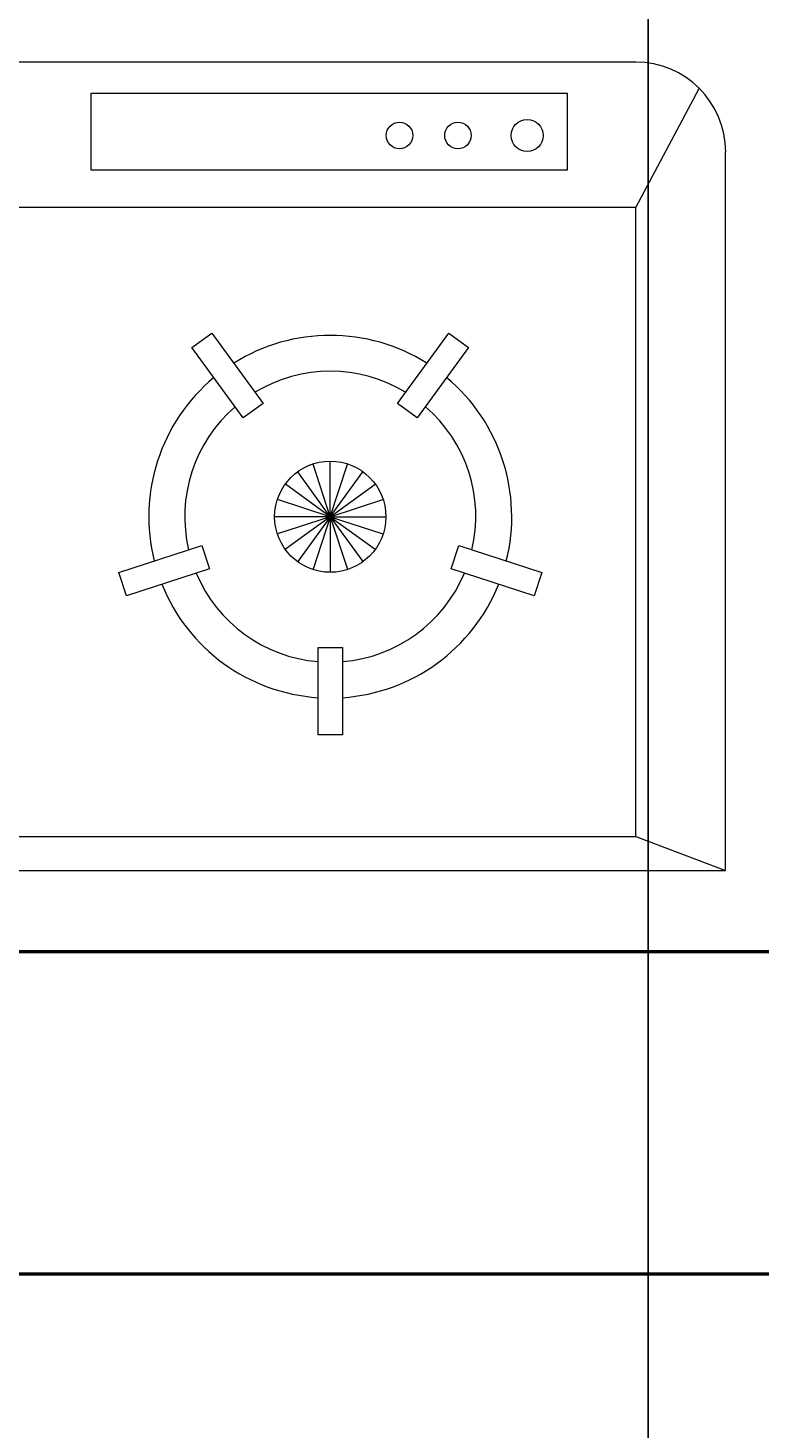
# Model space of a CAD drawing. Units: inches. Extents: x -173 to 545, y -746 to 104.
# Tile 5 of 32: x 203 to 223, y -702 to -663. Entities that reach past the tile are written whole.
import ezdxf

# ---------------------------------------------------------------- set-up
doc = ezdxf.new("R2010")
doc.units = ezdxf.units.IN
doc.header["$MEASUREMENT"] = 0
for name, color, linetype, lineweight in [('A-ANNO-DIMS', 2, 'Continuous', 18), ('A-EQPM', 8, 'Continuous', 18), ('A-WALL', 7, 'Continuous', 50)]:
    doc.layers.add(name, color=color, linetype=linetype, lineweight=lineweight)
doc.styles.get("Standard").update_dxf_attribs({"font": 'arial.ttf'})
doc.dimstyles.get("Standard").update_dxf_attribs({"dimtxt": 0.18, "dimasz": 0.18, "dimexe": 0.18, "dimexo": 0.0625, "dimgap": 0.09, "dimtad": 0, "dimtih": 1, "dimtoh": 1, "dimdec": 0, "dimzin": 0, "dimdsep": 46, "dimlunit": 3, "dimtxsty": 'Standard', "dimcen": 0.09, "dimadec": 0, "dimazin": 0, "dimtfac": 1, "dimtdec": 0, "dimtofl": 0, "dimtmove": 0, "dimatfit": 3, "dimfxl": 1, "dimtolj": 1, "dimtzin": 0, "dimarcsym": 0})

# ---------------------------------------------------------------- blocks, each defined once
blk = doc.blocks.new('HOB-40-BURNER')
for p, q in [((2.04, 10.813), (2.594, 11.215)), ((2.594, 11.215), (4.025, 9.246)), ((7.767, 9.246), (9.198, 11.215)), ((9.198, 11.215), (9.752, 10.813)), ((3.471, 8.844), (2.04, 10.813)), ((9.752, 10.813), (8.321, 8.844)), ((4.025, 9.246), (3.471, 8.844)), ((8.321, 8.844), (7.767, 9.246)), ((5.896, 6.088), (5.419, 7.557)), ((5.896, 6.088), (5.896, 7.633)), ((5.896, 6.088), (6.373, 7.557)), ((5.896, 6.088), (4.988, 7.338)), ((5.896, 6.088), (6.804, 7.338)), ((5.896, 6.088), (4.647, 6.996)), ((5.896, 6.088), (7.145, 6.996)), ((5.896, 6.088), (4.428, 6.566)), ((5.896, 6.088), (7.365, 6.566)), ((5.896, 6.088), (4.352, 6.088)), ((5.896, 6.088), (4.428, 5.611)), ((5.896, 6.088), (4.647, 5.181)), ((5.896, 6.088), (4.988, 4.839)), ((5.896, 6.088), (5.419, 4.62)), ((5.896, 6.088), (7.44, 6.088)), ((5.896, 6.088), (7.365, 5.611)), ((5.896, 6.088), (7.145, 5.181)), ((5.896, 6.088), (6.804, 4.839)), ((5.896, 6.088), (6.373, 4.62)), ((5.896, 6.088), (5.896, 4.544)), ((0, 4.532), (2.315, 5.285)), ((2.315, 5.285), (2.527, 4.634)), ((9.266, 4.634), (9.477, 5.285)), ((9.477, 5.285), (11.792, 4.532)), ((0.211, 3.882), (0, 4.532)), ((2.527, 4.634), (0.211, 3.882)), ((11.581, 3.882), (9.266, 4.634)), ((11.792, 4.532), (11.581, 3.882)), ((5.554, 2.434), (6.238, 2.434)), ((5.554, 0), (5.554, 2.434)), ((6.238, 2.434), (6.238, 0)), ((6.238, 0), (5.554, 0))]:
    blk.add_line(p, q)
blk.add_circle((5.896, 6.088), 1.551)
for radius, start, end in [(5.061, 57.8765, 122.1235), (5.061, 129.8765, 194.1235), (4.058, 58.8365, 121.1635), (5.061, 345.8765, 50.1235), (4.058, 130.8365, 193.1635), (4.058, 346.8365, 49.1635), (4.058, 202.8365, 265.1635), (4.058, 274.8365, 337.1635), (5.061, 201.8765, 266.1235), (5.061, 273.8765, 338.1235)]:
    blk.add_arc((5.896, 6.088), radius, start, end)
blk = doc.blocks.new('*D81')
at = {"layer": 'A-ANNO-DIMS', "color": 0, "lineweight": -2, "transparency": 16777216}
for p, q in [((219.801, -551.924), (219.801, -740.642)), ((306.301, -551.924), (306.301, -740.642)), ((219.981, -740.462), (262.513, -740.462)), ((306.121, -740.462), (263.59, -740.462))]:
    blk.add_line(p, q, dxfattribs=at)
at = {"layer": 'A-ANNO-DIMS', "color": 0, "transparency": 16777216}
for points in [[(219.981, -740.432), (219.981, -740.492), (219.801, -740.462)], [(306.121, -740.432), (306.121, -740.492), (306.301, -740.462)]]:
    blk.add_solid(points, dxfattribs=at)
at = {"layer": 'Defpoints', "color": 0, "transparency": 16777216}
for p in [(219.801, -551.862), (306.301, -551.862), (306.301, -740.462)]:
    blk.add_point(p, dxfattribs=at)
at = {"layer": 'A-ANNO-DIMS', "color": 0, "transparency": 16777216, "insert": (263.051, -740.462), "char_height": 0.18, "attachment_point": 5}
blk.add_mtext('\\A1;7\'-2 1/2"', dxfattribs=at)

msp = doc.modelspace()

# ---------------------------------------------------------------- linework, layer by layer
at = {"layer": 'A-EQPM'}
for p, q in [((219.455, -663.545), (184.36, -663.545)), ((204.268, -664.408), (217.538, -664.408)), ((204.268, -666.557), (204.268, -664.408)), ((217.538, -664.408), (217.538, -666.557)), ((219.455, -667.606), (221.227, -664.279)), ((221.961, -686.106), (221.961, -666.052)), ((217.538, -666.557), (204.268, -666.557)), ((219.455, -667.606), (184.36, -667.606)), ((219.455, -685.154), (219.455, -667.606)), ((184.36, -685.154), (219.455, -685.154)), ((219.455, -685.154), (221.961, -686.106)), ((181.854, -686.106), (221.961, -686.106))]:
    msp.add_line(p, q, dxfattribs=at)
for centre, radius in [((212.867, -665.593), 0.37), ((214.498, -665.593), 0.37), ((216.426, -665.593), 0.445)]:
    msp.add_circle(centre, radius, dxfattribs=at)
msp.add_arc((219.455, -666.052), 2.507, 0, 90, dxfattribs=at)
at = {"layer": 'A-WALL'}
for p, q in [((169.801, -688.362), (260.801, -688.362)), ((24.301, -697.362), (501.801, -697.362))]:
    msp.add_line(p, q, dxfattribs=at)

# ---------------------------------------------------------------- block references
at = {"layer": 'A-EQPM'}
msp.add_blockref('HOB-40-BURNER', (205.041, -682.32), dxfattribs=at)

# ---------------------------------------------------------------- dimensions: what is measured, and where the dimension line sits
at = {"layer": 'A-ANNO-DIMS'}
dim = msp.add_linear_dim(base=(306.301, -740.462), p1=(219.801, -551.862), p2=(306.301, -551.862), dimstyle='Standard', override={"dimdec": 1, "dimlfac": 1, "dimrnd": 0, "dimzin": 1, "dimdsep": 46, "dimlunit": 4, "dimfrac": 2}, dxfattribs=at)
dim.commit()
dim.dimension.update_dxf_attribs({"geometry": '*D81', "text_midpoint": (263.051, -740.462)})

doc.saveas('drawing.dxf')
